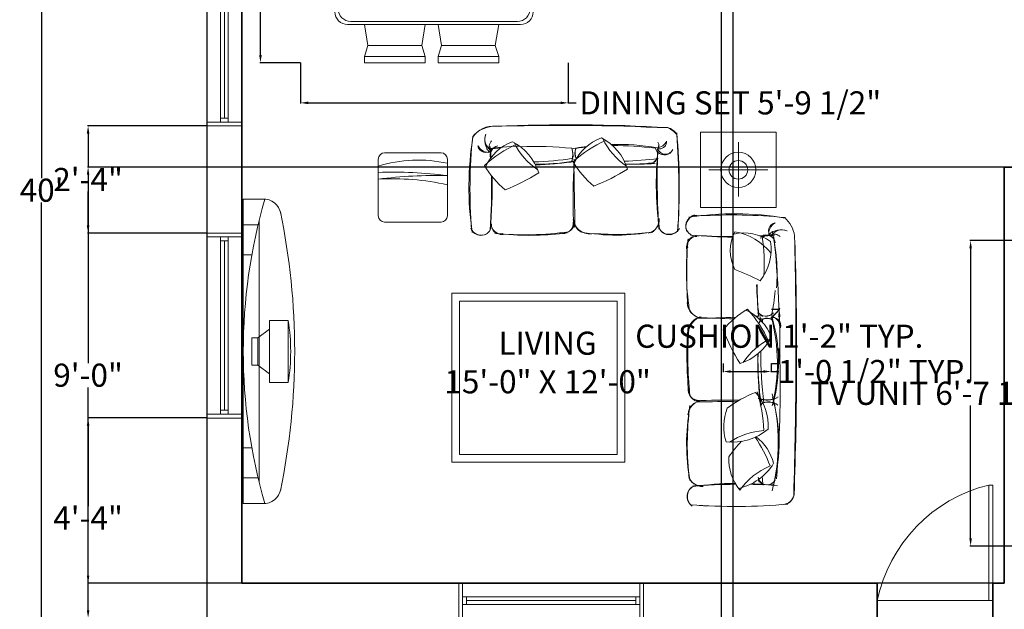
# Model space of a CAD drawing. Units: inches. Extents: x 84 to 590, y 32 to 648.
# Tile 2 of 6: x 84 to 340, y 248 to 401. Entities that reach past the tile are written whole.
import ezdxf

# ---------------------------------------------------------------- set-up
doc = ezdxf.new("R2010")
doc.units = ezdxf.units.IN
doc.header["$MEASUREMENT"] = 0
for name, color, linetype, lineweight in [('A-ANNO-DIMS', 2, 'Continuous', 18), ('A-AREA-IDEN', 7, 'Continuous', 18), ('A-DOOR', 4, 'Continuous', 18), ('A-FURN', 8, 'Continuous', 18), ('A-GLAZ', 4, 'Continuous', 18), ('A-WALL', 7, 'Continuous', 35), ('C-PROP', 7, 'Continuous', 30)]:
    doc.layers.add(name, color=color, linetype=linetype, lineweight=lineweight)
doc.styles.get("Standard").update_dxf_attribs({"font": 'arial.ttf'})
doc.dimstyles.get("Standard").update_dxf_attribs({"dimtxt": 6, "dimasz": 2, "dimexe": 0.18, "dimexo": 0.0625, "dimgap": 0.09, "dimtad": 0, "dimtih": 1, "dimtoh": 1, "dimdec": 0, "dimzin": 0, "dimdsep": 46, "dimlunit": 4, "dimtxsty": 'Standard', "dimcen": 0.09, "dimadec": 0, "dimazin": 0, "dimtfac": 1, "dimtdec": 0, "dimtofl": 0, "dimtmove": 0, "dimatfit": 3, "dimfxl": 1, "dimtolj": 1, "dimtzin": 0, "dimarcsym": 1})

# ---------------------------------------------------------------- blocks, each defined once
blk = doc.blocks.new('DOOR')
for p, q in [((185.51, 1128.53), (185.51, 1098.53)), ((185.51, 1128.53), (186.51, 1128.53)), ((186.51, 1098.53), (186.51, 1128.53)), ((186.51, 1098.53), (156.51, 1098.53))]:
    blk.add_line(p, q)
blk.add_arc((194.73, 1090.6), 39.03, 103.6607, 168.2814)
blk = doc.blocks.new('A$C78AE5658')
for p, q in [((1515, 306), (1515, 524)), ((1515, 524), (2236, 524)), ((2236, 306), (2236, 524)), ((98, 250), (98, 252)), ((98, 250), (98, 0)), ((1515, 306), (2236, 306)), ((1613, 306), (1716, 168)), ((2137, 306), (2034, 168)), ((3648, 250), (3648, 252)), ((3648, 0), (3648, 250)), ((348, 184), (3398, 184)), ((398, 0), (398, 172)), ((2034, 168), (1716, 168)), ((1716, 168), (1716, 98)), ((2034, 168), (2034, 98)), ((3348, 0), (3348, 172)), ((3648, 0), (98, 0)), ((748, 0), (748, 99)), ((2034, 98), (1716, 98)), ((2998, 0), (2998, 99))]:
    blk.add_line(p, q)
blk.add_lwpolyline([(246, 432, -0.103184), (3500, 432, -0.103184)], format="xyb")
for centre, radius, start, end in [((1875, -1675), 2228, 80.6925, 99.3075), ((298, 239), 200, 98.4687, 183.693), ((3449, 239), 200, 356.307, 81.5313), ((1873, 6426), 6426, 253.9658, 286.0342)]:
    blk.add_arc(centre, radius, start, end)
blk = doc.blocks.new('A$C6C037A94')
for p, q in [((0.7877, 1.6959), (0.4032, 1.6959)), ((0.4032, 1.6959), (0.4039, 1.6557)), ((0.7877, 1.6557), (0.7877, 1.6959)), ((0.4258, 1.588), (0.4039, 1.6557)), ((0.7877, 1.6557), (0.4039, 1.6557)), ((0.7658, 1.588), (0.7877, 1.6557)), ((0.407, 1.4737), (0.4258, 1.588)), ((0.7658, 1.588), (0.4258, 1.588)), ((0.7847, 1.4737), (0.7658, 1.588)), ((0.307, 1.4737), (0.8868, 1.4737)), ((0.327, 1.4537), (0.8668, 1.4537)), ((0.227, 0.2974), (0.227, 1.3937)), ((0.247, 0.3174), (0.247, 1.3737)), ((0.9468, 1.3737), (0.9468, 0.3174)), ((0.9668, 1.3937), (0.9668, 0.2974)), ((0, 1.2552), (0, 0.8707)), ((0.0402, 1.2552), (0, 1.2552)), ((0.0402, 1.2552), (0.0402, 0.8714)), ((0.1079, 1.2333), (0.0402, 1.2552)), ((0.227, 1.2529), (0.1079, 1.2333)), ((0.9668, 1.2553), (1.1005, 1.2333)), ((1.1005, 1.2333), (1.1682, 1.2552)), ((1.1682, 1.2552), (1.2084, 1.2552)), ((1.1682, 1.2552), (1.1682, 0.8714)), ((1.2084, 1.2552), (1.2084, 0.8707)), ((0.1079, 1.2333), (0.1079, 0.8933)), ((1.1005, 1.2333), (1.1005, 0.8933)), ((0.1079, 0.8933), (0.0402, 0.8714)), ((0.227, 0.8736), (0.1079, 0.8933)), ((0.9668, 0.8712), (1.1005, 0.8933)), ((1.1005, 0.8933), (1.1682, 0.8714)), ((0, 0.8707), (0.0402, 0.8714)), ((1.2084, 0.8707), (1.1682, 0.8714)), ((0, 0.7888), (0, 0.4043)), ((0.0402, 0.7888), (0, 0.7888)), ((0.0402, 0.7888), (0.0402, 0.405)), ((0.1079, 0.7669), (0.0402, 0.7888)), ((0.227, 0.7865), (0.1079, 0.7669)), ((0.1079, 0.7669), (0.1079, 0.4269)), ((0.9668, 0.7889), (1.1005, 0.7669)), ((1.1005, 0.7669), (1.1682, 0.7888)), ((1.1005, 0.7669), (1.1005, 0.4269)), ((1.1682, 0.7888), (1.1682, 0.405)), ((1.1682, 0.7888), (1.2084, 0.7888)), ((1.2084, 0.7888), (1.2084, 0.4043)), ((0, 0.4043), (0.0402, 0.405)), ((0.1079, 0.4269), (0.0402, 0.405)), ((0.227, 0.4072), (0.1079, 0.4269)), ((0.9668, 0.4048), (1.1005, 0.4269)), ((1.1005, 0.4269), (1.1682, 0.405)), ((1.2084, 0.4043), (1.1682, 0.405)), ((0.8868, 0.2174), (0.307, 0.2174)), ((0.8668, 0.2374), (0.327, 0.2374)), ((0.4078, 0.2174), (0.4258, 0.1079)), ((0.7839, 0.2174), (0.7658, 0.1079)), ((0.4258, 0.1079), (0.4039, 0.0402)), ((0.7658, 0.1079), (0.4258, 0.1079)), ((0.7658, 0.1079), (0.7877, 0.0402)), ((0.4032, 0), (0.4039, 0.0402)), ((0.7877, 0), (0.4032, 0)), ((0.7877, 0.0402), (0.4039, 0.0402)), ((0.7877, 0.0402), (0.7877, 0))]:
    blk.add_line(p, q)
for centre, start, end in [((0.307, 1.3937), 90, 180), ((0.327, 1.3737), 90, 180), ((0.8668, 1.3737), 360, 90), ((0.8868, 1.3937), 360, 90), ((0.327, 0.3174), 180, 270), ((0.8668, 0.3174), 270, 0), ((0.307, 0.2974), 180, 270), ((0.8868, 0.2974), 270, 360)]:
    blk.add_arc(centre, 0.08, start, end)
blk = doc.blocks.new('*D13')
at = {"layer": 'A-ANNO-DIMS', "color": 0, "lineweight": -2, "transparency": 16777216}
for p, q in [((132.97, 608.34), (89.87, 608.34)), ((90.05, 606.34), (90.05, 359.49)), ((90.05, 106.34), (90.05, 353.18)), ((132.97, 104.34), (89.87, 104.34))]:
    blk.add_line(p, q, dxfattribs=at)
at = {"layer": 'A-ANNO-DIMS', "color": 0, "transparency": 16777216}
for points in [[(89.71, 606.34), (90.38, 606.34), (90.05, 608.34)], [(89.71, 106.34), (90.38, 106.34), (90.05, 104.34)]]:
    blk.add_solid(points, dxfattribs=at)
at = {"layer": 'Defpoints', "color": 0, "transparency": 16777216}
for p in [(90.05, 608.34), (133.03, 608.34), (133.03, 104.34)]:
    blk.add_point(p, dxfattribs=at)
at = {"layer": 'A-ANNO-DIMS', "color": 0, "transparency": 16777216, "insert": (90.05, 356.34), "char_height": 6, "attachment_point": 5}
blk.add_mtext("\\A1;40'", dxfattribs=at)
blk = doc.blocks.new('WIND')
for p, q in [((-51.89, 1021.98), (-99.89, 1021.98)), ((-99.89, 1021.98), (-99.89, 1012.98)), ((-98.89, 1021.98), (-98.89, 1012.98)), ((-52.89, 1012.98), (-52.89, 1021.98)), ((-51.89, 1012.98), (-51.89, 1021.98)), ((-98.89, 1018.48), (-52.89, 1018.48)), ((-97.89, 1018.48), (-97.89, 1016.48)), ((-53.89, 1016.48), (-53.89, 1018.48)), ((-98.89, 1016.48), (-52.89, 1016.48)), ((-97.89, 1017.48), (-53.89, 1017.48)), ((-99.89, 1012.98), (-51.89, 1012.98))]:
    blk.add_line(p, q)
blk = doc.blocks.new('FURN-THROW-PILLOW')
for centre, radius, start, end in [((18.24, -6.3), 23.62, 120.3068, 140.5663), ((1.13, 2.76), 12.05, 19.4501, 66.7699), ((-17.28, -7.37), 31.9, 24.0815, 42.2768), ((47.08, 27.1), 50.54, 201.3371, 212.4176), ((0.46, 12.91), 13.5, 287.0126, 332.9429), ((20.26, -10.05), 18.27, 115.9005, 145.6513)]:
    blk.add_arc(centre, radius, start, end)
blk = doc.blocks.new('*D25')
at = {"layer": 'A-ANNO-DIMS', "color": 0, "lineweight": -2, "transparency": 16777216}
for p, q in [((343.11, 343.29), (331.1, 343.29)), ((331.28, 341.29), (331.28, 306.83)), ((331.28, 265.98), (331.28, 300.44)), ((343.11, 263.98), (331.1, 263.98))]:
    blk.add_line(p, q, dxfattribs=at)
at = {"layer": 'A-ANNO-DIMS', "color": 0, "transparency": 16777216}
for points in [[(330.95, 341.29), (331.61, 341.29), (331.28, 343.29)], [(330.95, 265.98), (331.61, 265.98), (331.28, 263.98)]]:
    blk.add_solid(points, dxfattribs=at)
at = {"layer": 'Defpoints', "color": 0, "transparency": 16777216}
for p in [(343.17, 343.29), (331.28, 263.98), (343.17, 263.98)]:
    blk.add_point(p, dxfattribs=at)
at = {"layer": 'A-ANNO-DIMS', "color": 0, "transparency": 16777216, "insert": (331.28, 303.64), "char_height": 6, "attachment_point": 5}
blk.add_mtext('\\A1;TV UNIT 6\'-7 1/2" TYP.', dxfattribs=at)
blk = doc.blocks.new('*D31')
at = {"layer": 'A-ANNO-DIMS', "color": 0, "lineweight": -2, "transparency": 16777216}
for p, q in [((157.31, 389.37), (157.31, 378.83)), ((226.82, 389.37), (226.82, 378.83)), ((159.31, 379.01), (224.82, 379.01)), ((226.82, 379.01), (228.82, 379.01))]:
    blk.add_line(p, q, dxfattribs=at)
at = {"layer": 'A-ANNO-DIMS', "color": 0, "transparency": 16777216}
for points in [[(159.31, 379.34), (159.31, 378.67), (157.31, 379.01)], [(224.82, 379.34), (224.82, 378.67), (226.82, 379.01)]]:
    blk.add_solid(points, dxfattribs=at)
at = {"layer": 'Defpoints', "color": 0, "transparency": 16777216}
for p in [(157.31, 389.43), (226.82, 389.43), (226.82, 379.01)]:
    blk.add_point(p, dxfattribs=at)
at = {"layer": 'A-ANNO-DIMS', "color": 0, "transparency": 16777216, "insert": (268.87, 379.01), "char_height": 6, "attachment_point": 5}
blk.add_mtext('\\A1;DINING SET 5\'-9 1/2"', dxfattribs=at)
blk = doc.blocks.new('*D32')
at = {"layer": 'A-ANNO-DIMS', "color": 0, "lineweight": -2, "transparency": 16777216}
for p, q in [((157.25, 438.96), (146.7, 438.96)), ((146.88, 436.96), (146.88, 417.39)), ((146.88, 391.43), (146.88, 411)), ((157.25, 389.43), (146.7, 389.43))]:
    blk.add_line(p, q, dxfattribs=at)
at = {"layer": 'A-ANNO-DIMS', "color": 0, "transparency": 16777216}
for points in [[(146.55, 436.96), (147.22, 436.96), (146.88, 438.96)], [(146.55, 391.43), (147.22, 391.43), (146.88, 389.43)]]:
    blk.add_solid(points, dxfattribs=at)
at = {"layer": 'Defpoints', "color": 0, "transparency": 16777216}
for p in [(157.31, 438.96), (146.88, 389.43), (157.31, 389.43)]:
    blk.add_point(p, dxfattribs=at)
at = {"layer": 'A-ANNO-DIMS', "color": 0, "transparency": 16777216, "insert": (146.88, 414.2), "char_height": 6, "attachment_point": 5}
blk.add_mtext('\\A1;4\'-1 1/2"', dxfattribs=at)
blk = doc.blocks.new('*D41')
at = {"layer": 'A-ANNO-DIMS', "color": 0, "lineweight": -2, "transparency": 16777216}
for p, q in [((279.55, 325.5), (281.78, 325.5)), ((281.6, 323.5), (281.6, 321.64)), ((281.6, 313.4), (281.6, 315.25)), ((279.55, 311.4), (281.78, 311.4))]:
    blk.add_line(p, q, dxfattribs=at)
at = {"layer": 'A-ANNO-DIMS', "color": 0, "transparency": 16777216}
for points in [[(281.27, 323.5), (281.94, 323.5), (281.6, 325.5)], [(281.27, 313.4), (281.94, 313.4), (281.6, 311.4)]]:
    blk.add_solid(points, dxfattribs=at)
at = {"layer": 'Defpoints', "color": 0, "transparency": 16777216}
for p in [(279.49, 325.5), (281.6, 325.5), (279.49, 311.4)]:
    blk.add_point(p, dxfattribs=at)
at = {"layer": 'A-ANNO-DIMS', "color": 0, "transparency": 16777216, "insert": (281.6, 318.45), "char_height": 6, "attachment_point": 5}
blk.add_mtext('\\A1;CUSHION 1\'-2" TYP.', dxfattribs=at)
blk = doc.blocks.new('*D42')
at = {"layer": 'A-ANNO-DIMS', "color": 0, "lineweight": -2, "transparency": 16777216}
for p, q in [((267.01, 311.34), (267.01, 309.11)), ((279.49, 311.34), (279.49, 309.11)), ((269.01, 309.29), (277.49, 309.29)), ((279.49, 309.29), (281.49, 309.29))]:
    blk.add_line(p, q, dxfattribs=at)
at = {"layer": 'A-ANNO-DIMS', "color": 0, "transparency": 16777216}
for points in [[(269.01, 309.62), (269.01, 308.95), (267.01, 309.29)], [(277.49, 309.62), (277.49, 308.95), (279.49, 309.29)]]:
    blk.add_solid(points, dxfattribs=at)
at = {"layer": 'Defpoints', "color": 0, "transparency": 16777216}
for p in [(267.01, 311.4), (279.49, 311.4), (279.49, 309.29)]:
    blk.add_point(p, dxfattribs=at)
at = {"layer": 'A-ANNO-DIMS', "color": 0, "transparency": 16777216, "insert": (306.57, 309.29), "char_height": 6, "attachment_point": 5}
blk.add_mtext('\\A1;1\'-0 1/2" TYP.', dxfattribs=at)
blk = doc.blocks.new('*D53')
at = {"layer": 'A-ANNO-DIMS', "color": 0, "lineweight": -2, "transparency": 16777216}
for p, q in [((132.97, 297.23), (101.95, 297.23)), ((102.13, 295.23), (102.13, 274.37)), ((102.13, 247.34), (102.13, 268.19)), ((141.97, 245.34), (101.95, 245.34))]:
    blk.add_line(p, q, dxfattribs=at)
at = {"layer": 'A-ANNO-DIMS', "color": 0, "transparency": 16777216}
for points in [[(101.79, 295.23), (102.46, 295.23), (102.13, 297.23)], [(101.79, 247.34), (102.46, 247.34), (102.13, 245.34)]]:
    blk.add_solid(points, dxfattribs=at)
at = {"layer": 'Defpoints', "color": 0, "transparency": 16777216}
for p in [(102.13, 297.23), (133.03, 297.23), (142.03, 245.34)]:
    blk.add_point(p, dxfattribs=at)
at = {"layer": 'A-ANNO-DIMS', "color": 0, "transparency": 16777216, "insert": (102.13, 271.28), "char_height": 6, "attachment_point": 5}
blk.add_mtext('\\A1;4\'-4"', dxfattribs=at)
blk = doc.blocks.new('*D54')
at = {"layer": 'A-ANNO-DIMS', "color": 0, "lineweight": -2, "transparency": 16777216}
for p, q in [((132.97, 373.02), (101.95, 373.02)), ((102.13, 371.02), (102.13, 362.23)), ((102.13, 347.23), (102.13, 356.02)), ((132.97, 345.23), (101.95, 345.23))]:
    blk.add_line(p, q, dxfattribs=at)
at = {"layer": 'A-ANNO-DIMS', "color": 0, "transparency": 16777216}
for points in [[(101.79, 371.02), (102.46, 371.02), (102.13, 373.02)], [(101.79, 347.23), (102.46, 347.23), (102.13, 345.23)]]:
    blk.add_solid(points, dxfattribs=at)
at = {"layer": 'Defpoints', "color": 0, "transparency": 16777216}
for p in [(102.13, 373.02), (133.03, 373.02), (133.03, 345.23)]:
    blk.add_point(p, dxfattribs=at)
at = {"layer": 'A-ANNO-DIMS', "color": 0, "transparency": 16777216, "insert": (102.13, 359.12), "char_height": 6, "attachment_point": 5}
blk.add_mtext('\\A1;2\'-4"', dxfattribs=at)
blk = doc.blocks.new('*D61')
at = {"layer": 'A-ANNO-DIMS', "color": 0, "lineweight": -2, "transparency": 16777216}
for p, q in [((339.97, 362.34), (101.95, 362.34)), ((102.13, 360.34), (102.13, 311.49)), ((102.13, 256.34), (102.13, 305.18)), ((339.97, 254.34), (101.95, 254.34))]:
    blk.add_line(p, q, dxfattribs=at)
at = {"layer": 'A-ANNO-DIMS', "color": 0, "transparency": 16777216}
for points in [[(101.79, 360.34), (102.46, 360.34), (102.13, 362.34)], [(101.79, 256.34), (102.46, 256.34), (102.13, 254.34)]]:
    blk.add_solid(points, dxfattribs=at)
at = {"layer": 'Defpoints', "color": 0, "transparency": 16777216}
for p in [(102.13, 362.34), (340.03, 362.34), (340.03, 254.34)]:
    blk.add_point(p, dxfattribs=at)
at = {"layer": 'A-ANNO-DIMS', "color": 0, "transparency": 16777216, "insert": (102.13, 308.34), "char_height": 6, "attachment_point": 5}
blk.add_mtext('\\A1;9\'-0"', dxfattribs=at)
blk = doc.blocks.new('*D63')
at = {"layer": 'A-ANNO-DIMS', "color": 0, "lineweight": -2, "transparency": 16777216}
for p, q in [((266.53, 450.78), (266.53, 73.26)), ((269.53, 450.78), (269.53, 73.26)), ((264.53, 73.44), (262.53, 73.44)), ((271.53, 73.44), (273.53, 73.44))]:
    blk.add_line(p, q, dxfattribs=at)
at = {"layer": 'A-ANNO-DIMS', "color": 0, "transparency": 16777216}
for points in [[(264.53, 73.77), (264.53, 73.1), (266.53, 73.44)], [(271.53, 73.77), (271.53, 73.1), (269.53, 73.44)]]:
    blk.add_solid(points, dxfattribs=at)
at = {"layer": 'Defpoints', "color": 0, "transparency": 16777216}
for p in [(266.53, 450.84), (269.53, 450.84), (269.53, 73.44)]:
    blk.add_point(p, dxfattribs=at)
at = {"layer": 'A-ANNO-DIMS', "color": 0, "transparency": 16777216, "insert": (281.59, 73.44), "char_height": 6, "attachment_point": 5}
blk.add_mtext('\\A1;0\'-3"', dxfattribs=at)

msp = doc.modelspace()

# ---------------------------------------------------------------- linework, layer by layer
at = {"layer": 'A-DOOR'}
msp.add_line((337.03, 279.84), (336.03, 279.84), dxfattribs=at)
at = {"layer": 'A-FURN'}
for p, q in [((261.17, 351.83), (261.17, 371.44)), ((261.17, 371.44), (280.78, 371.44)), ((280.78, 371.44), (280.78, 351.83)), ((270.98, 361.63), (270.98, 368.79)), ((193.79, 366.04), (179.08, 366.04)), ((177.44, 364.41), (177.44, 349.7)), ((195.42, 349.7), (195.42, 364.41)), ((270.98, 361.63), (263.32, 361.63)), ((270.98, 361.63), (270.98, 354.74)), ((270.98, 361.63), (278.63, 361.63)), ((182.53, 359.7), (182.53, 359.7)), ((280.78, 351.83), (261.17, 351.83)), ((179.08, 348.06), (193.79, 348.06)), ((258.88, 278.91), (258.88, 278.91)), ((258.88, 278.91), (258.88, 278.91)), ((259.02, 280.75), (259.02, 280.75)), ((273.1, 279.46), (273.1, 279.46)), ((273.59, 279.42), (273.59, 279.42))]:
    msp.add_line(p, q, dxfattribs=at)
for points in [[(196.58, 329.59), (241.51, 329.59), (241.51, 285.78), (196.58, 285.78)], [(198.58, 327.59), (239.51, 327.59), (239.51, 287.78), (198.58, 287.78)]]:
    msp.add_lwpolyline(points, close=True, dxfattribs=at)
for radius in [4.56, 2.41]:
    msp.add_circle((270.98, 361.63), radius, dxfattribs=at)
for centre, radius, start, end in [((226.92, -71.88), 445.21, 86.6876, 92.4329), ((207.34, 366.58), 6.39, 83.8792, 147.1093), ((207.87, 365.15), 7.81, 98.6549, 138.7104), ((208.16, 369.61), 3.04, 154.8715, 246.7247), ((209.96, 369.35), 4.8, 161.2473, 221.1348), ((224.93, -211.32), 584.48, 87.2697, 91.7875), ((251.5, 368.62), 4.13, 31.8817, 73.9672), ((249.07, 365.19), 8.19, 43.5462, 63.1435), ((108.23, 357.26), 147.41, 355.4325, 5.431), ((39.16, 355.96), 216.36, 357.3143, 3.933), ((282.23, 357.18), 81.22, 170.8079, 188.3514), ((333.31, 356.65), 132.02, 174.0627, 184.6253), ((208.7, 367.51), 2.43, 137.7203, 204.4461), ((239.58, 309.36), 58.88, 79.9466, 91.5903), ((333.97, 358), 84.31, 172.9836, 187.989), ((249.77, 370.12), 2.74, 271.184, 337.8216), ((248.8, 367.92), 1.55, 314.3938, 33.5856), ((250.51, 368.88), 1.81, 268.0108, 6.5585), ((179.08, 364.41), 1.63, 90, 180), ((193.79, 364.41), 1.63, 0, 90), ((206.14, 369.3), 3.13, 207.8433, 279.8684), ((205.4, 368.17), 2.06, 189.2916, 317.6289), ((217.31, 285.92), 81.95, 92.2017, 98.3067), ((218.06, 268.92), 98.78, 95.0871, 96.7491), ((208.56, 365.44), 2.07, 147.7366, 202.2387), ((86.97, 357.09), 120.07, 3.7101, 5.0653), ((60.96, 356.57), 145.94, 3.1908, 3.7892), ((208.94, 365.57), 2.31, 100.6216, 199.193), ((218.06, 268.92), 98.78, 84.3639, 92.1219), ((221.22, 365.56), 6.75, 344.0479, 14.2061), ((222.5, 365.46), 5.55, 351.5362, 18.3493), ((239.03, 292.17), 75.75, 95.7795, 98.522), ((231.24, 365.87), 2.73, 149.8319, 209.468), ((232.59, 366.07), 4.02, 163.3108, 202.6164), ((239.58, 309.36), 58.88, 97.803, 100.4557), ((239.03, 292.17), 75.75, 82.1551, 90.5585), ((247.61, 365.57), 2.41, 276.1174, 43.1189), ((438.88, 359.24), 188.98, 177.5073, 183.9592), ((252.02, 367.7), 2.05, 194.7814, 337.5922), ((251.79, 367.79), 2.3, 222.3134, 337.6102), ((187.86, 328.84), 35.31, 77.6304, 107.1636), ((216.69, 431.45), 67.76, 271.0061, 279.6001), ((217.44, 454.04), 90.97, 270.4949, 276.3291), ((216.23, 435.22), 72.35, 271.6458, 279.5268), ((236.15, 336.02), 28.94, 105.9625, 107.4638), ((242.61, 504.11), 141.03, 263.8872, 264.1215), ((354.32, 354.1), 126.28, 175.8425, 183.2873), ((229.71, 365.22), 1.71, 209.1313, 222.0141), ((-1439704.39, -25319.37), 1440161.66, 1.02115803, 1.02184547), ((354.32, 354.1), 126.28, 175.3655, 175.4784), ((239.37, 446.71), 82.85, 262.7245, 262.7726), ((239.37, 446.71), 82.85, 271.3731, 277.4472), ((242.61, 504.11), 141.03, 269.6386, 272.7653), ((240.26, 476.45), 113.41, 270.7456, 274.456), ((248.07, 365.24), 1.91, 257.6226, 350.3094), ((181.14, 249.18), 111.85, 82.6617, 91.8937), ((192.38, 240.85), 119.31, 88.539, 97.1936), ((181.15, 294.23), 65.09, 77.3313, 93.2642), ((60.96, 356.57), 145.94, 355.8027, 1.3803), ((86.97, 357.09), 120.07, 354.7422, 1.3335), ((279.29, 343.88), 6.39, 56.0023, 56.0023), ((179.08, 349.7), 1.63, 180, 270), ((193.79, 349.7), 1.63, 270, 0), ((209.84, 347.95), 3.14, 177.6579, 284.0974), ((225.38, 347.83), 2.75, 252.9316, 5.1092), ((225.72, 348.02), 2.73, 253.4437, 1.8228), ((232.35, 349.27), 4.26, 186.5867, 283.4511), ((231.56, 348.28), 3.11, 174.9234, 245.6374), ((246.91, 348.7), 3.54, 280.9756, 4.9747), ((247.01, 348.37), 3.27, 289.8228, 2.4985), ((260, 347.1), 2.7, 71.3412, 252.8428), ((260.62, 346.86), 3.26, 108.7066, 202.6723), ((269.88, 268.99), 81.22, 80.6341, 98.3514), ((269.35, 217.91), 132.02, 84.0627, 93.6881), ((280.87, 345.82), 2.06, 99.2916, 227.6289), ((282, 345.08), 3.13, 117.8433, 189.8684), ((277.85, 343.35), 7.81, 8.6549, 48.7104), ((204.12, 347.3), 2.7, 197.7157, 342.8428), ((204.36, 347.92), 3.26, 216.0678, 292.6723), ((209.05, 347.16), 2.18, 170.2617, 291.0115), ((215.48, 430.15), 85.38, 264.8245, 277.7148), ((216.81, 416.93), 72.3, 265.0781, 277.695), ((239.27, 398.55), 53.85, 260.0543, 280.4167), ((239.35, 416.77), 71.9, 265.2072, 277.551), ((253.06, 347.69), 2.89, 194.6379, 334.3095), ((253.06, 347.96), 3.08, 213.041, 316.0653), ((279.24, 340.7), 10.38, 152.1942, 208.1227), ((272.39, 333.19), 12.05, 54.6654, 102.5832), ((267.81, 331.05), 14.66, 37.4475, 81.1735), ((282.06, 341.26), 4.8, 71.2473, 131.1348), ((282.31, 343.06), 3.04, 64.8715, 156.7247), ((233.02, 334.57), 48.01, 355.7167, 13.4699), ((330.36, 335.71), 72.87, 173.7078, 188.1597), ((260.65, 341.38), 3.14, 87.6579, 186.5963), ((401.29, 334.76), 143.72, 176.538, 183.2518), ((259.86, 342.17), 2.18, 80.2617, 201.0115), ((269.27, 490.26), 145.94, 265.8027, 270.0952), ((269.79, 464.24), 120.07, 264.7422, 269.8415), ((269.27, 490.26), 145.94, 272.8469, 273.7892), ((265.99, 341.1), 13.5, 322.2037, 8.1582), ((407.07, 336.37), 130.47, 176.6143, 176.7488), ((269.79, 464.24), 120.07, 273.3663, 275.0653), ((278.14, 342.97), 1.82, 52.2499, 131.1322), ((234.53, 337.26), 43.17, 355.9091, 9.3319), ((278.49, 342.51), 2.07, 5.5094, 125.3618), ((280.21, 342.51), 2.43, 47.7203, 114.4461), ((-7.96, 314.01), 289.73, 359.6375, 5.9901), ((-963.31, 315.27), 1249.23, 358.2517, 1.34182), ((-684.99, 313.22), 971.09, 357.87913, 1.76902), ((231.22, 241.19), 102.29, 63.6226, 67.6678), ((360.32, 334), 84.63, 181.5276, 186.7252), ((436.06, 333.76), 160.22, 180.6743, 183.6481), ((226.72, 334.55), 53.97, 348.572, 355.4817), ((261.58, 327.19), 3.9, 180.2562, 250.009), ((262.14, 327.43), 4.42, 190.7326, 248.8706), ((278.13, 326.2), 2.55, 213.6302, 319.4072), ((273.33, 330.68), 9.71, 311.3239, 329.6489), ((278.22, 327.3), 3.81, 294.9311, 336.316), ((263.98, 317.96), 6.32, 118.8275, 183.1679), ((262.05, 319.36), 4.2, 99.6723, 190.8758), ((258.2, 602.42), 279.3, 270.3569, 272.4781), ((273.63, 563.31), 240.36, 266.8793, 269.0887), ((258.2, 602.42), 279.3, 273.5599, 273.9253), ((278.11, 326.84), 3.15, 229.246, 304.576), ((278.33, 320.96), 2.21, 42.6233, 153.9248), ((273.63, 563.31), 240.36, 270.6475, 270.7982), ((278.43, 320.12), 2.94, 58.0934, 131.8441), ((378.02, 312.11), 102, 173.6313, 174.0106), ((357.57, 312.32), 81.51, 172.3637, 172.7445), ((407.07, 336.37), 130.47, 185.514, 185.6423), ((367.15, 313.29), 90.35, 173.8205, 174.432), ((279.95, 321.23), 2.06, 341.7747, 110.1119), ((234, 311.44), 47.11, 346.4246, 14.6799), ((239.95, 311.71), 41.45, 344.5471, 16.7487), ((278.77, 320.57), 3.13, 0.3263, 72.3514), ((357.6, 313.51), 99.98, 175.6872, 184.822), ((358.11, 313.42), 100.27, 175.4063, 185.976), ((367.15, 313.29), 90.35, 179.1949, 187.7065), ((378.02, 312.11), 102, 179.0125, 185.4293), ((357.57, 312.32), 81.51, 178.887, 188.2861), ((-3.54, 305.29), 285.39, 355.2123, 1.384), ((260.67, 304.55), 2.75, 168.429, 275.1092), ((260.87, 304.21), 2.73, 163.4437, 271.8228), ((262.11, 297.57), 4.26, 96.5867, 173.3659), ((266.95, 175.61), 126.28, 88.0798, 93.2873), ((286.55, 275.31), 30.65, 111.2126, 127.0845), ((265.69, 295.23), 13.05, 356.0508, 41.5115), ((243.04, 293.08), 34.56, 1.5034, 18.4401), ((278.3, 307.42), 5.55, 246.4473, 302.7025), ((248.86, 293.78), 28.94, 13.524, 17.4638), ((278.41, 308.7), 6.75, 254.0479, 292.8429), ((354.39, 290.18), 78.61, 171.1063, 171.8048), ((231.97, 290.9), 49.37, 345.2542, 14.7458), ((239.68, 290.64), 41.86, 345.3745, 16.5383), ((311.39, 290.65), 53.85, 170.0543, 190.4167), ((329.61, 290.58), 71.9, 172.0869, 187.551), ((261.12, 298.37), 3.11, 103.3965, 179.8407), ((-25406.53, 1440234.31), 1440161.66, 271.02119422, 271.02160701), ((280.04, 295.01), 12.87, 158.3873, 197.8438), ((278.71, 298.69), 2.73, 47.9567, 138.0859), ((266.95, 175.61), 126.28, 85.3655, 85.3663), ((278.91, 297.33), 4.02, 54.1749, 112.4749), ((269.4, 305.61), 14.62, 263.6702, 309.5436), ((279.21, 274.26), 19.79, 94.7049, 122.2519), ((247.29, 272.98), 34.04, 20.3191, 34.4817), ((267.72, 282.17), 12.85, 14.8665, 52.3615), ((293.5, 270.23), 30.18, 136.0462, 145.9003), ((281.16, 286.53), 12.67, 177.2031, 219.1005), ((267.88, 293.02), 14.4, 282.4859, 328.3594), ((286.98, 266.92), 19.49, 113.5207, 143.4241), ((261.54, 283.01), 3.54, 190.9756, 274.9747), ((261.21, 282.91), 3.27, 199.8228, 272.4985), ((389.29, 289.67), 113.41, 183.9965, 184.456), ((354.39, 290.18), 78.61, 186.1109, 186.9851), ((278.41, 282.31), 2.41, 205.1742, 332.9234), ((278.08, 281.85), 1.91, 196.7712, 260.3094), ((359.55, 290.55), 82.85, 185.932, 187.4472), ((260.5, 276.87), 2.87, 115.1873, 227.995), ((260.81, 276.86), 3.08, 113.6813, 233.9016), ((272.09, 91.05), 188.98, 90.5455, 93.9592), ((270.84, 195.95), 84.31, 90.4744, 97.884), ((272.09, 91.05), 188.98, 87.5073, 89.3973), ((270.84, 195.95), 84.31, 82.9836, 87.5705), ((282.35, 277.92), 3.14, 273.9909, 348.3328), ((282.58, 277.5), 2.78, 282.8701, 352.7992), ((270.16, 423.11), 148.83, 265.5341, 275.2764), ((267.35, 490.77), 216.36, 268.2528, 268.8905)]:
    msp.add_arc(centre, radius, start, end, dxfattribs=at)
at = {"layer": 'A-WALL'}
for p, q in [((142.03, 254.34), (142.03, 446.34)), ((382.03, 362.34), (340.03, 362.34)), ((340.03, 254.34), (340.03, 362.34)), ((142.03, 254.34), (307.03, 254.34)), ((307.03, 245.34), (307.03, 254.34)), ((337.03, 245.34), (337.03, 254.34)), ((337.03, 254.34), (340.03, 254.34))]:
    msp.add_line(p, q, dxfattribs=at)
at = {"layer": 'C-PROP'}
msp.add_line((133.03, 104.34), (133.03, 608.34), dxfattribs=at)

# ---------------------------------------------------------------- block references
at = {"layer": 'A-DOOR'}
msp.add_blockref('DOOR', (150.52, -848.69), dxfattribs=at)
at = {"layer": 'A-FURN', "rotation": 270}
for name, p, xscale, yscale, zscale in [('A$C6C037A94', (157.31, 438.96), 40.98563321974356, 40.98563321974356, 40.98563321974356), ('A$C78AE5658', (142.43, 356.21), 0.0222542726180731, 0.0222542726180731, 0.0222542726180731)]:
    msp.add_blockref(name, p, dxfattribs=dict(at, xscale=xscale, yscale=yscale, zscale=zscale))
at = {"layer": 'A-FURN'}
for p, rotation in [((219.13, 356.43), 90.00000000162429), ((242.17, 357.42), 90.00000000162179)]:
    msp.add_blockref('FURN-THROW-PILLOW', p, dxfattribs=dict(at, rotation=rotation))
msp.add_blockref('FURN-THROW-PILLOW', (267.01, 311.4), dxfattribs=at)
at = {"layer": 'A-GLAZ', "rotation": 270}
for p in [(-879.95, 321.13), (-879.95, 245.33)]:
    msp.add_blockref('WIND', p, dxfattribs=at)
at = {"layer": 'A-GLAZ'}
msp.add_blockref('WIND', (298.25, -767.64), dxfattribs=at)

# ---------------------------------------------------------------- texts
at = {"layer": 'A-AREA-IDEN', "insert": (148.84, 319.64), "char_height": 6, "attachment_point": 1}
msp.add_mtext_dynamic_manual_height_columns('\\pxqc;LIVING\\P15\'-0" X 12\'-0"', width=145.2094, gutter_width=30, heights=[0], dxfattribs=at)

# ---------------------------------------------------------------- dimensions: what is measured, and where the dimension line sits
at = {"layer": 'A-ANNO-DIMS'}
for base, p1, p2, angle, text, override, picture, middle in [((90.05, 608.34), (133.03, 104.34), (133.03, 608.34), 90, "40'", {"dimclrd": 0, "dimclre": 0, "dimclrt": 0}, '*D13', (90.05, 356.34)), ((331.28, 263.98), (343.17, 343.29), (343.17, 263.98), 270, 'TV UNIT <> TYP.', {"dimdec": 1, "dimlfac": 1, "dimrnd": 0, "dimzin": 1, "dimdsep": 46, "dimlunit": 4, "dimfrac": 2}, '*D25', (331.28, 303.64)), ((281.6, 325.5), (279.49, 311.4), (279.49, 325.5), 90, 'CUSHION <> TYP.', {"dimdec": 1, "dimlfac": 1, "dimrnd": 0, "dimzin": 1, "dimdsep": 46, "dimlunit": 4, "dimfrac": 2}, '*D41', (281.6, 318.45))]:
    dim = msp.add_linear_dim(base=base, p1=p1, p2=p2, angle=angle, text=text, dimstyle='Standard', override=override, dxfattribs=at)
    dim.commit()
    dim.dimension.update_dxf_attribs({"geometry": picture, "text_midpoint": middle})
dim = msp.add_linear_dim(base=(269.53, 73.44), p1=(266.53, 450.84), p2=(269.53, 450.84), dimstyle='Standard', override={"dimdec": 1, "dimlfac": 1, "dimrnd": 0, "dimzin": 1, "dimdsep": 46, "dimlunit": 4, "dimfrac": 2}, dxfattribs=at)
dim.commit()
dim.dimension.update_dxf_attribs({"geometry": '*D63', "text_midpoint": (281.59, 73.44)})
for base, p1, p2, angle, picture, middle in [((146.88, 389.43), (157.31, 438.96), (157.31, 389.43), 270, '*D32', (146.88, 414.2)), ((102.13, 373.02), (133.03, 345.23), (133.03, 373.02), 90, '*D54', (102.13, 359.12)), ((102.13, 362.34), (340.03, 254.34), (340.03, 362.34), 90, '*D61', (102.13, 308.34)), ((102.13, 297.23), (142.03, 245.34), (133.03, 297.23), 90, '*D53', (102.13, 271.28))]:
    dim = msp.add_linear_dim(base=base, p1=p1, p2=p2, angle=angle, dimstyle='Standard', override={"dimdec": 1, "dimlfac": 1, "dimrnd": 0, "dimzin": 1, "dimdsep": 46, "dimlunit": 4, "dimfrac": 2}, dxfattribs=at)
    dim.commit()
    dim.dimension.update_dxf_attribs({"geometry": picture, "text_midpoint": middle})
for base, p1, p2, text, picture, middle in [((226.82, 379.01), (157.31, 389.43), (226.82, 389.43), 'DINING SET <>', '*D31', (268.87, 379.01)), ((279.49, 309.29), (267.01, 311.4), (279.49, 311.4), '<> TYP.', '*D42', (306.57, 309.29))]:
    dim = msp.add_linear_dim(base=base, p1=p1, p2=p2, text=text, dimstyle='Standard', override={"dimdec": 1, "dimlfac": 1, "dimrnd": 0, "dimzin": 1, "dimdsep": 46, "dimlunit": 4, "dimfrac": 2}, dxfattribs=at)
    dim.commit()
    dim.dimension.update_dxf_attribs({"geometry": picture, "text_midpoint": middle})

doc.saveas('drawing.dxf')
